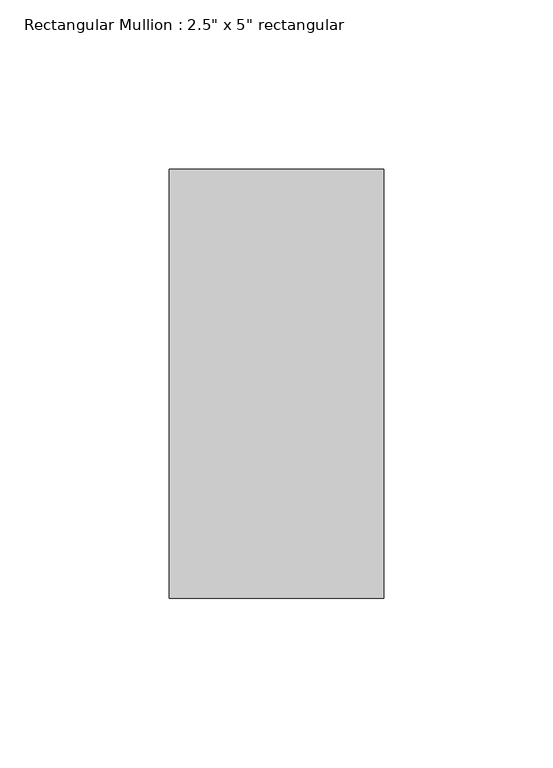
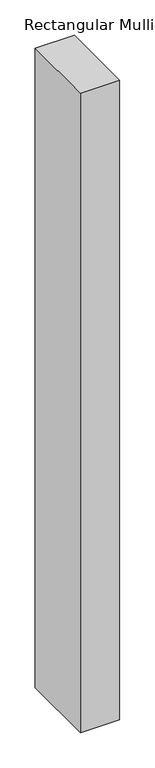
"""IFC4 building model written with IfcOpenShell, lengths in millimetres: member geometry."""

from ifc_helpers import new_model, si_unit, frame, origin, place, context, project, spatial, polyline, outline, extrude, source, transform, mapped, element, save


def member_b90701c7(model_context):
    return source(origin(), model_context, "Body", "SweptSolid", [
        extrude(outline(polyline([(31.75, 63.5), (31.75, -63.5), (-31.75, -63.5), (-31.75, 63.5), (31.75, 63.5)])), frame((0.0, 0.0, -1099.5770399), z_axis=(0.0, 0.0, 1.0), x_axis=(1.0, 0.0, 0.0)), (0.0, 0.0, 1.0), 1099.5770399),
    ])


if __name__ == "__main__":
    model = new_model("IFC4")
    model_context = context("Model", 3, world=origin())
    ifc_project = project(units=[si_unit("LENGTHUNIT", "METRE", prefix="MILLI")], contexts=[model_context])
    site = spatial("IfcSite", under=ifc_project)
    building = spatial("IfcBuilding", under=site)
    placement = place(None, origin())
    member_shape = member_b90701c7(model_context)
    element("IfcMember", 1, ObjectType="Rectangular Mullion : 2.5\" x 5\" rectangular", at=placement, inside=building, context=model_context, shape_type="MappedRepresentation", body=[
        mapped(member_shape, transform((0.0, 0.0, 0.0), x_axis=(1.0, 0.0, 0.0), y_axis=(0.0, 1.0, 0.0), z_axis=(0.0, 0.0, 1.0))),
    ])
    save(model, "model.ifc")

# Revit data of these elements
# Type "Rectangular Mullion : 2.5\" x 5\" rectangular"
#   built-in parameter 1007304 = 0.416667 (stored number, unit not read)
#   built-in parameter 1007301 = 0.104167 (stored number, unit not read)
#   built-in parameter 1007300 = 0.104167 (stored number, unit not read)
# Element 1 (IfcMember, "Rectangular Mullion : 2.5\" x 5\" rectangular")
#   Materials on its faces: "Aluminum"
# Materials
#   "Aluminum": class "Metal", colour RGB 247 247 247, transparency 0, Description = "Aluminum 6061", Cost = 0
